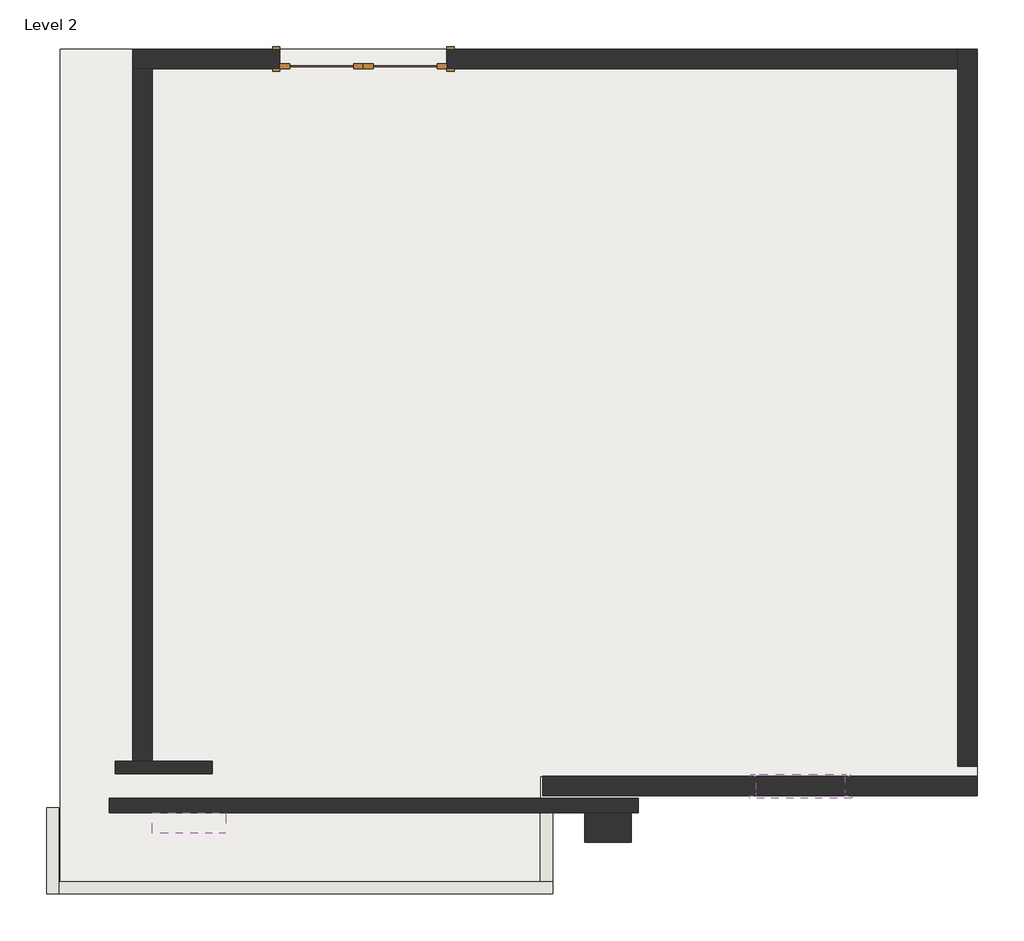
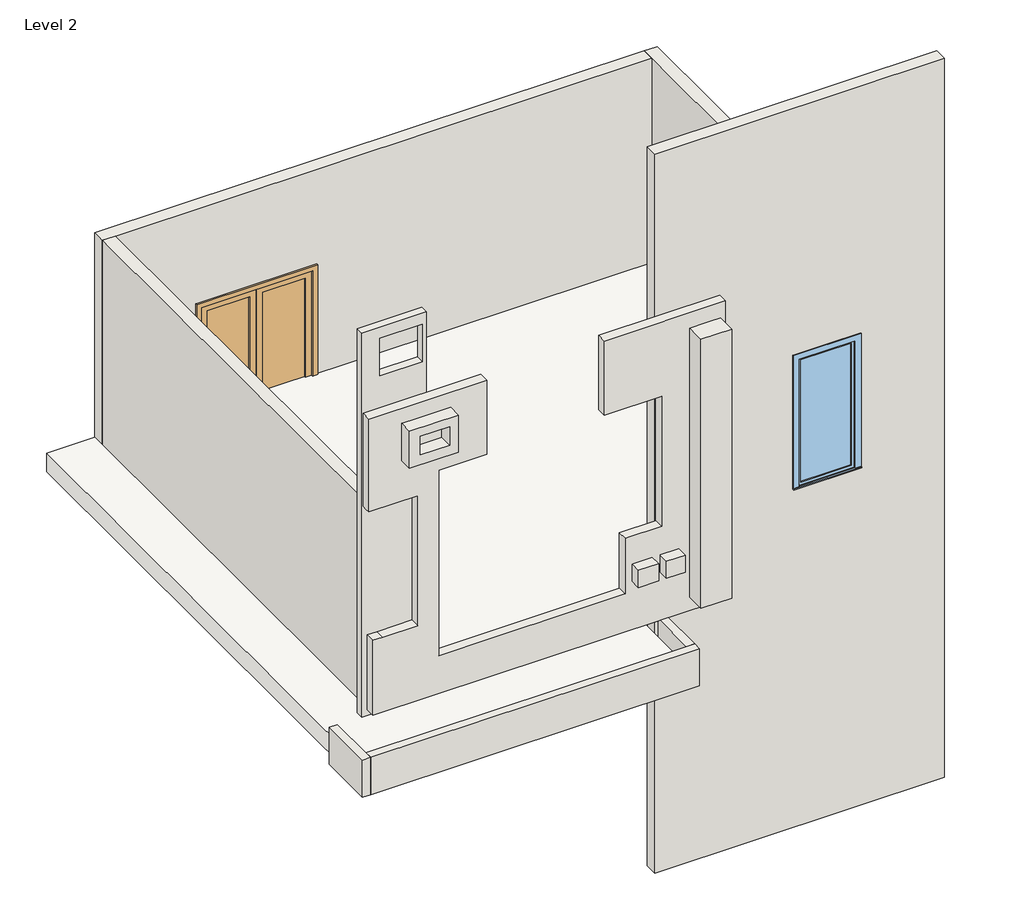
# One storey: 11 walls, 1 door, 1 roof, 1 window.
"""IFC4 building model written with IfcOpenShell, lengths in millimetres."""

from ifc_helpers import new_model, si_unit, frame, origin, place, context, project, spatial, polyline, outline, extrude, faceted_brep, transform, mapped, element, save
from components import door_10418eaf, walls_2_walls_2_2f288bc8, walls_4_walls_4_9e78723f, window_4ca78fb8

model = new_model("IFC4")

# Units and contexts
model_context = context("Model", 3, world=origin())
ifc_project = project(units=[si_unit("LENGTHUNIT", "METRE", prefix="MILLI")], contexts=[model_context])

# Site, building, storey
site = spatial("IfcSite", under=ifc_project)
building = spatial("IfcBuilding", under=site)
storey = spatial("IfcBuildingStorey", under=building, Name="Level 2", Elevation=3657.6)

# Door
placement = place(None, origin())
door_shape = door_10418eaf(model_context)
element("IfcDoor", 1, ObjectType="Door-Double-Glass : 68\" x 80\"", at=placement, inside=storey, context=model_context, shape_type="MappedRepresentation", body=[
    mapped(door_shape, transform((-7523.7093643, 9433.1639635, 3657.6), x_axis=(-1.0, 0.0, 0.0), y_axis=(0.0, -1.0, 0.0), z_axis=(0.0, 0.0, 1.0))),
])

# Roof
element("IfcRoof", 2, ObjectType="Generic - 12\"", at=placement, inside=storey, context=model_context, shape_type="SweptSolid", body=[
    extrude(outline(polyline([(-9911.3093643, 9532.3827135), (-1173.7093643, 9532.3827135), (-1173.7093643, 2013.9827135), (-5694.9093643, 2013.9827135), (-5694.9093643, 921.7827135), (-10660.6093643, 921.7827135), (-10660.6093643, 9532.3827135), (-9911.3093643, 9532.3827135)])), frame((0.0, 0.0, 3657.6), z_axis=(0.0, 0.0, 1.0), x_axis=(1.0, 0.0, 0.0)), (0.0, 0.0, 1.0), 304.8),
])

# Walls
element("IfcWall", 3, ObjectType="Generic - 5\"", at=placement, inside=storey, context=model_context, shape_type="Brep", body=[
    faceted_brep([(-10800.3093643, 1683.7827135, 3657.6), (-10800.3093643, 794.7827135, 3657.6), (-10800.3093643, 794.7827135, 4267.2), (-10800.3093643, 1683.7827135, 4267.2), (-10673.3093643, 1683.7827135, 3657.6), (-10673.3093643, 1683.7827135, 4267.2), (-10673.3093643, 921.7827135, 4267.2), (-10673.3093643, 794.7827135, 4267.2), (-10673.3093643, 794.7827135, 3657.6), (-10673.3093643, 921.7827135, 3657.6)], [[[0, 1, 2, 3]], [[4, 5, 6, 7, 8, 9]], [[1, 0, 4, 9, 8]], [[3, 2, 7, 6, 5]], [[0, 3, 5, 4]], [[2, 1, 8, 7]]]),
])
element("IfcWall", 4, ObjectType="Generic - 5\"", at=placement, inside=storey, context=model_context, shape_type="Brep", body=[
    faceted_brep([(-10673.3093643, 794.7827135, 3657.6), (-5567.9093643, 794.7827135, 3657.6), (-5567.9093643, 794.7827135, 4267.2), (-10673.3093643, 794.7827135, 4267.2), (-10673.3093643, 921.7827135, 3657.6), (-10673.3093643, 921.7827135, 4267.2), (-5694.9093643, 921.7827135, 4267.2), (-5567.9093643, 921.7827135, 4267.2), (-5567.9093643, 921.7827135, 3657.6), (-5694.9093643, 921.7827135, 3657.6)], [[[0, 1, 2, 3]], [[4, 5, 6, 7, 8, 9]], [[1, 0, 4, 9, 8]], [[3, 2, 7, 6, 5]], [[0, 3, 5, 4]], [[2, 1, 8, 7]]]),
])
element("IfcWall", 5, ObjectType="Generic - 5\"", at=placement, inside=storey, context=model_context, shape_type="SweptSolid", body=[
    extrude(outline(polyline([(-5567.9093643, 1683.7827135), (-5567.9093643, 921.7827135), (-5694.9093643, 921.7827135), (-5694.9093643, 1683.7827135), (-5567.9093643, 1683.7827135)])), frame((0.0, 0.0, 3657.6), z_axis=(0.0, 0.0, 1.0), x_axis=(1.0, 0.0, 0.0)), (0.0, 0.0, 1.0), 609.6),
])
element("IfcWall", 6, ObjectType="Generic - 5\"", at=placement, inside=storey, context=model_context, shape_type="SweptSolid", body=[
    extrude(outline(polyline([(3966.5333662, -10089.1093643), (3966.5333662, -9085.8093643), (10273.3442045, -9085.8093643), (10273.3442045, -10089.1093643), (3966.5333662, -10089.1093643)]), holes=[polyline([(10088.7905157, -9149.3093643), (9479.1905157, -9149.3093643), (9479.1905157, -9809.7093643), (10088.7905157, -9809.7093643), (10088.7905157, -9149.3093643)])]), frame((0.0, 2039.3827135, 0.0), z_axis=(0.0, 1.0, 0.0), x_axis=(0.0, 0.0, 1.0)), (0.0, 0.0, 1.0), 127.0),
])
element("IfcWall", 7, ObjectType="Generic - 6\"", at=placement, inside=storey, context=model_context, shape_type="Brep", body=[
    faceted_brep([(-4678.9093643, 1632.9827135, 4267.2), (-4678.9093643, 1632.9827135, 9154.5573397), (-6558.5093643, 1632.9827135, 9154.5573397), (-6558.5093643, 1632.9827135, 7936.9342302), (-5669.5093643, 1632.9827135, 7936.9342302), (-5669.5093643, 1632.9827135, 5803.3342302), (-6235.0832287, 1632.9827135, 5803.3342302), (-6235.0832287, 1632.9827135, 4888.9342302), (-9130.6832287, 1632.9827135, 4888.9342302), (-9130.6832287, 1632.9827135, 7936.9342302), (-8387.3093643, 1632.9827135, 7936.9342302), (-8387.3093643, 1632.9827135, 9154.5573397), (-10216.1093643, 1632.9827135, 9154.5573397), (-10216.1093643, 1632.9827135, 7630.5573397), (-9454.1093643, 1632.9827135, 7630.5573397), (-9454.1093643, 1632.9827135, 5496.9573397), (-10000.2093643, 1632.9827135, 5496.9573397), (-10152.6093643, 1632.9827135, 5496.9573397), (-10152.6093643, 1632.9827135, 4267.2), (-4678.9093643, 1785.3827135, 4267.2), (-10152.6093643, 1785.3827135, 4267.2), (-10152.6093643, 1785.3827135, 5496.9573397), (-10000.2093643, 1785.3827135, 5496.9573397), (-9454.1093643, 1785.3827135, 5496.9573397), (-9454.1093643, 1785.3827135, 7630.5573397), (-10089.1093643, 1785.3827135, 7630.5573397), (-10216.1093643, 1785.3827135, 7630.5573397), (-10216.1093643, 1785.3827135, 8872.1089518), (-10216.1093643, 1785.3827135, 9154.5573397), (-8387.3093643, 1785.3827135, 9154.5573397), (-8387.3093643, 1785.3827135, 7936.9342302), (-9130.6832287, 1785.3827135, 7936.9342302), (-9130.6832287, 1785.3827135, 4888.9342302), (-6235.0832287, 1785.3827135, 4888.9342302), (-6235.0832287, 1785.3827135, 5803.3342302), (-5669.5093643, 1785.3827135, 5803.3342302), (-5669.5093643, 1785.3827135, 7936.9342302), (-6558.5093643, 1785.3827135, 7936.9342302), (-6558.5093643, 1785.3827135, 9154.5573397), (-4678.9093643, 1785.3827135, 9154.5573397), (-10216.1093643, 1709.1827135, 7630.5573397)], [[[0, 1, 2, 3, 4, 5, 6, 7, 8, 9, 10, 11, 12, 13, 14, 15, 16, 17, 18]], [[19, 20, 21, 22, 23, 24, 25, 26, 27, 28, 29, 30, 31, 32, 33, 34, 35, 36, 37, 38, 39]], [[0, 18, 20, 19]], [[1, 0, 19, 39]], [[14, 13, 40, 26, 25, 24]], [[15, 14, 24, 23]], [[16, 15, 23, 22]], [[17, 16, 22, 21]], [[18, 17, 21, 20]], [[9, 8, 32, 31]], [[5, 4, 36, 35]], [[8, 7, 33, 32]], [[6, 5, 35, 34]], [[7, 6, 34, 33]], [[2, 1, 39, 38]], [[3, 2, 38, 37]], [[4, 3, 37, 36]], [[10, 9, 31, 30]], [[11, 10, 30, 29]], [[12, 11, 29, 28]], [[13, 12, 28, 27, 26, 40]]]),
])
element("IfcWall", 8, ObjectType="Generic - 8\"", at=placement, inside=storey, context=model_context, shape_type="Brep", body=[
    faceted_brep([(-9911.3093643, 9329.1827135, 3657.6), (-9708.1093643, 9329.1827135, 3657.6), (-8387.3093643, 9329.1827135, 3657.6), (-8387.3093643, 9329.1827135, 5689.6), (-6660.1093643, 9329.1827135, 5689.6), (-6660.1093643, 9329.1827135, 3657.6), (-1376.9093643, 9329.1827135, 3657.6), (-1376.9093643, 9329.1827135, 7315.2), (-9708.1093643, 9329.1827135, 7315.2), (-9911.3093643, 9329.1827135, 7315.2), (-8387.3093643, 9532.3827135, 5689.6), (-8387.3093643, 9532.3827135, 3657.6), (-9911.3093643, 9532.3827135, 3657.6), (-9911.3093643, 9532.3827135, 7315.2), (-1376.9093643, 9532.3827135, 7315.2), (-1376.9093643, 9532.3827135, 3657.6), (-6660.1093643, 9532.3827135, 3657.6), (-6660.1093643, 9532.3827135, 5689.6)], [[[0, 1, 2, 3, 4, 5, 6, 7, 8, 9]], [[10, 11, 12, 13, 14, 15, 16, 17]], [[16, 15, 6, 5]], [[12, 11, 2, 1, 0]], [[9, 8, 7, 14, 13]], [[0, 9, 13, 12]], [[7, 6, 15, 14]], [[3, 2, 11, 10]], [[4, 3, 10, 17]], [[5, 4, 17, 16]]]),
])
element("IfcWall", 9, ObjectType="Generic - 8\"", at=placement, inside=storey, context=model_context, shape_type="SweptSolid", body=[
    extrude(outline(polyline([(-9708.1093643, 9329.1827135), (-9708.1093643, 2166.3827135), (-9911.3093643, 2166.3827135), (-9911.3093643, 9329.1827135), (-9708.1093643, 9329.1827135)])), frame((0.0, 0.0, 3657.6), z_axis=(0.0, 0.0, 1.0), x_axis=(1.0, 0.0, 0.0)), (0.0, 0.0, 1.0), 3657.6),
])
element("IfcWall", 10, ObjectType="Generic - 8\"", at=placement, inside=storey, context=model_context, shape_type="Brep", body=[
    faceted_brep([(-1376.9093643, 9532.3827135, 3657.6), (-1376.9093643, 9329.1827135, 3657.6), (-1376.9093643, 2115.5827135, 3657.6), (-1376.9093643, 2115.5827135, 7315.2), (-1376.9093643, 9329.1827135, 7315.2), (-1376.9093643, 9532.3827135, 7315.2), (-1173.7093643, 9532.3827135, 3657.6), (-1173.7093643, 9532.3827135, 7315.2), (-1173.7093643, 2115.5827135, 7315.2), (-1173.7093643, 2115.5827135, 3657.6)], [[[0, 1, 2, 3, 4, 5]], [[6, 7, 8, 9]], [[2, 1, 0, 6, 9]], [[3, 2, 9, 8]], [[5, 4, 3, 8, 7]], [[0, 5, 7, 6]]]),
])
element("IfcWall", 11, ObjectType="Generic - 8\"", at=placement, inside=storey, context=model_context, shape_type="Brep", body=[
    faceted_brep([(-5669.5093643, 1810.7827135, 0.0), (-1173.7093643, 1810.7827135, 0.0), (-1173.7093643, 1810.7827135, 11806.7857686), (-5669.5093643, 1810.7827135, 11806.7857686), (-3459.7093643, 1810.7827135, 7682.7861951), (-2545.3093643, 1810.7827135, 7682.7861951), (-2545.3093643, 1810.7827135, 5549.1861951), (-3459.7093643, 1810.7827135, 5549.1861951), (-5669.5093643, 2013.9827135, 0.0), (-5669.5093643, 2013.9827135, 7315.2), (-5669.5093643, 2013.9827135, 10967.8023446), (-5669.5093643, 2013.9827135, 11806.7857686), (-1173.7093643, 2013.9827135, 11806.7857686), (-1173.7093643, 2013.9827135, 10942.7791309), (-1173.7093643, 2013.9827135, 7315.2), (-1173.7093643, 2013.9827135, 0.0), (-3459.7093643, 2013.9827135, 7682.7861951), (-3459.7093643, 2013.9827135, 5549.1861951), (-2545.3093643, 2013.9827135, 5549.1861951), (-2545.3093643, 2013.9827135, 7682.7861951)], [[[0, 1, 2, 3], [4, 5, 6, 7]], [[8, 9, 10, 11, 12, 13, 14, 15], [16, 17, 18, 19]], [[1, 0, 8, 15]], [[3, 2, 12, 11]], [[2, 1, 15, 14, 13, 12]], [[0, 3, 11, 10, 9, 8]], [[17, 16, 4, 7]], [[18, 17, 7, 6]], [[19, 18, 6, 5]], [[16, 19, 5, 4]]]),
])
walls_2_walls_2_shape = walls_2_walls_2_2f288bc8(model_context)
element("IfcWall", 12, ObjectType="Walls 2 : Walls 2", at=placement, inside=storey, context=model_context, shape_type="MappedRepresentation", body=[
    mapped(walls_2_walls_2_shape, transform((0.0, 0.0, 0.0), x_axis=(1.0, 0.0, 0.0), y_axis=(0.0, 1.0, 0.0), z_axis=(0.0, 0.0, 1.0))),
])
walls_4_walls_4_shape = walls_4_walls_4_9e78723f(model_context)
element("IfcWall", 13, ObjectType="Walls 4 : Walls 4", at=placement, inside=storey, context=model_context, shape_type="MappedRepresentation", body=[
    mapped(walls_4_walls_4_shape, transform((0.0, 0.0, 0.0), x_axis=(1.0, 0.0, 0.0), y_axis=(0.0, 1.0, 0.0), z_axis=(0.0, 0.0, 1.0))),
])

# Window
window_shape = window_4ca78fb8(model_context)
element("IfcWindow", 14, ObjectType="Fixed with Trim : 36\" x 48\"", at=placement, inside=storey, context=model_context, shape_type="MappedRepresentation", body=[
    mapped(window_shape, transform((-3040.6093643, 1912.3827135, 4634.7861951), x_axis=(-1.0, 0.0, 0.0), y_axis=(0.0, -1.0, 0.0), z_axis=(0.0, 0.0, 1.0))),
])

save(model, "model.ifc")

# Revit data of these elements
# Type "Door-Double-Glass : 68\" x 80\""
#   Type Mark = "10"
#   Construction Type Id = "opn-d45"
#   Assembly Code = "C1020"
#   Analytic Construction = "Wood frame, double glass door "
#   W = 2' - 10"
#   Thickness = 0' - 2"
#   Thermal Resistance (R) = 1.8150 (h·ft²·°F)/BTU
#   Swing Angle [instance default] = 90.00°
#   Heat Transfer Coefficient (U) = 0.5510 BTU/(h·ft²·°F)
#   Height = 6' - 8"
#   Bottom Rail = 0' - 4"
#   Top Rail = 0' - 4"
#   Stiles = 0' - 4"
#   Trim Projection = 0' - 1"
#   Trim Width = 0' - 3"
#   Width = 5' - 8"
#   Define Thermal Properties by = 1
#   Glazing = Glass
#   Panel Material = Wood - Birch - Solid Stained Light Low Gloss
#   Trim Material = Paint - Sienna
#   Visual Light Transmittance = 0
#   Solar Heat Gain Coefficient = 0
#   Function = (empty or 0)
#   Wall Closure = (empty or 0)
# Type "Generic - 12\""
#   Assembly Code = "B1020"
#   Layers, outside or top first: 1' - 0" no material (function 1)
# Type "Generic - 5\""
#   Assembly Code = "B2010"
#   Layers, outside or top first: 0' - 5" no material (function 1)
# Type "Generic - 6\""
#   Assembly Code = "B2010"
#   Layers, outside or top first: 0' - 6" no material (function 1)
# Type "Generic - 8\""
#   Assembly Code = "B2010"
#   Layers, outside or top first: 0' - 8" no material (function 1)
# Type "Fixed with Trim : 36\" x 48\""
#   Type Mark = "10"
#   Construction Type Id = "GSP4R"
#   Assembly Code = "B2020100"
#   Analytic Construction = "1/8 in Pilkington single glazing"
#   Visual Light Transmittance = 0.9
#   Solar Heat Gain Coefficient = 0.78
#   Heat Transfer Coefficient (U) = 0.6496 BTU/(h·ft²·°F)
#   Height = 7' - 0"
#   Default Sill Height = 3' - 0"
#   Trim Projection - Ext. = 0' - 0 1/2"
#   Trim Projection - Int. = 0' - 0 3/4"
#   Trim Width - Exterior = 0' - 3 1/2"
#   Trim Width - Interior = 0' - 3 1/2"
#   Width = 3' - 0"
#   Window Inset = 0' - 0 3/4"
#   Define Thermal Properties by = 1
#   Glass Pane Material = Glass
#   Sash Material = Sash
#   Trim Exterior Material = Trim
#   Trim Interior Material = Trim
#   Wall Closure = (empty or 0)
# Element 1 (IfcDoor, "Door-Double-Glass : 68\" x 80\"")
#   Swing Angle = 90.00°
#   Phase Created = New Construction
#   Materials on its faces: "Wood - Birch - Solid Stained Light Low Gloss", "Paint - Sienna", "Glass"
# Element 2 (IfcRoof, "Generic - 12\"")
#   built-in parameter 1001705 = 13 (stored number, unit not read)
#   built-in parameter 1001710 = 33615
#   Phase Created = New Construction
#   Materials on its faces: "Default Roof"
# Elements 3, 4, 5 (IfcWall, "Generic - 5\"")
#   Top Offset = -10' - 0"
#   Base Offset = 0' - 0"
#   wall height = 2' - 0"
#   Phase Created = New Construction
#   Base Constraint = Level 2
#   Top Constraint = Level 3
#   Materials on its faces: "Default Wall"
# Element 6 (IfcWall, "Generic - 5\"")
#   built-in parameter 1001111 = 1' - 0.16273"
#   Top Offset = 9' - 8.46237"
#   Base Offset = 1' - 0.16273"
#   wall height = 20' - 8.29964"
#   Phase Created = New Construction
#   Base Constraint = Level 2
#   Top Constraint = Level 3
#   Materials on its faces: "Default Wall"
# Element 7 (IfcWall, "Generic - 6\"")
#   built-in parameter 1001111 = 2' - 0"
#   Top Offset = 0' - 0"
#   Base Offset = 2' - 0"
#   Unconnected Height = 16' - 0.41564"
#   wall height = 16' - 0.41564"
#   Phase Created = New Construction
#   Base Constraint = Level 2
#   Materials on its faces: "Default Wall"
# Elements 8, 9, 10 (IfcWall, "Generic - 8\"")
#   Top Offset = 0' - 0"
#   Base Offset = 0' - 0"
#   Unconnected Height = 12' - 0"
#   wall height = 12' - 0"
#   Phase Created = New Construction
#   Base Constraint = Level 2
#   Materials on its faces: "Default Wall"
# Element 11 (IfcWall, "Generic - 8\"")
#   built-in parameter 1001111 = -12' - 0"
#   Top Offset = 0' - 0"
#   Base Offset = -12' - 0"
#   Unconnected Height = 38' - 8.83409"
#   wall height = 38' - 8.83409"
#   Phase Created = New Construction
#   Base Constraint = Level 2
#   Materials on its faces: "Default Wall"
# Element 12 (IfcWall, "Walls 2 : Walls 2")
#   Phase Created = New Construction
#   Materials on its faces: "Default Wall"
# Element 13 (IfcWall, "Walls 4 : Walls 4")
#   Phase Created = New Construction
#   Materials on its faces: "Default Wall"
# Element 14 (IfcWindow, "Fixed with Trim : 36\" x 48\"")
#   Mark = "1"
#   Phase Created = New Construction
#   Materials on its faces: "Sash", "Trim", "Glass"
# Materials
#   "Glass": class "Glass", colour RGB 0 128 192, transparency 0.75, Description = "Soda Lime Glass", Cost = 0
#   "Wood - Birch - Solid Stained Light Low Gloss": class "Wood", colour RGB 210 159 95, transparency 0, Cost = 0
#   "Paint - Sienna": colour RGB 118 70 51, transparency 0, Cost = 0
#   "Sash": class "Wood", colour RGB 224 178 126, transparency 0
#   "Trim": class "Wood", colour RGB 224 178 126, transparency 0
#   "Default Roof": colour RGB 88 101 114, transparency 0
#   "Default Wall": colour RGB 128 128 128, transparency 0
